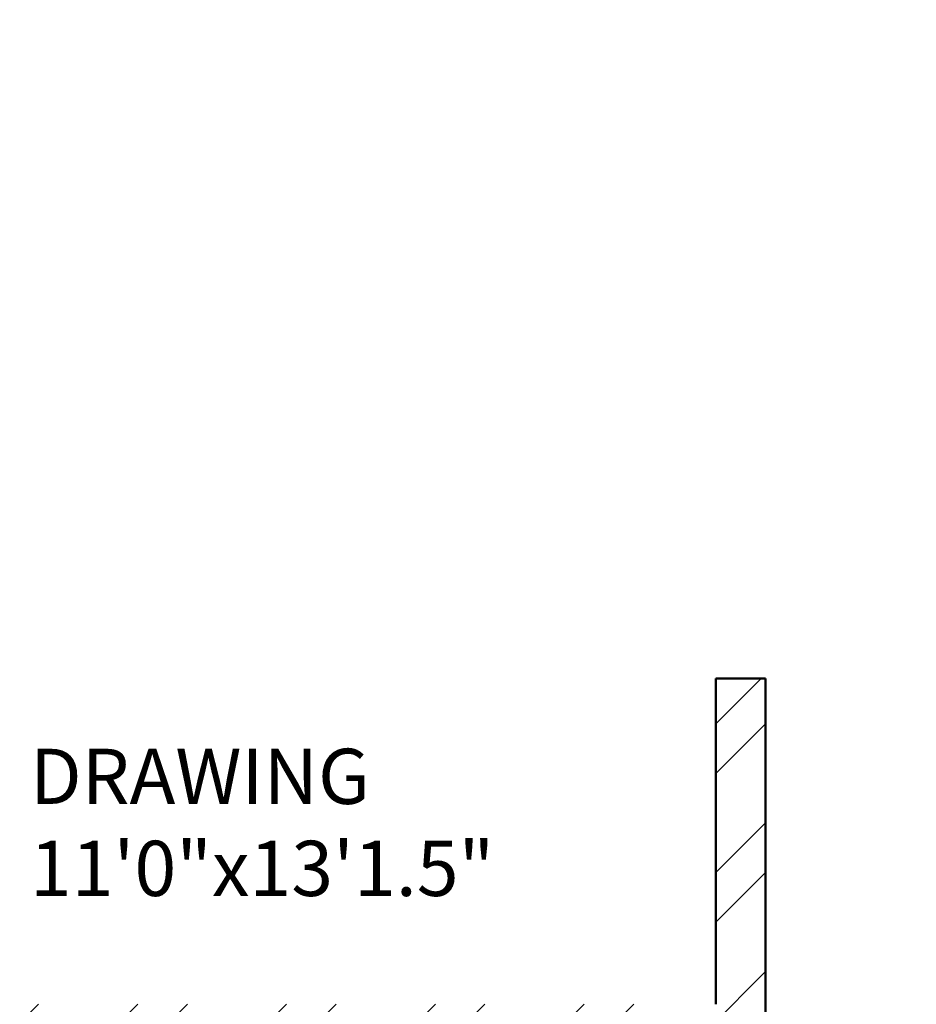
# Model space of a CAD drawing. Units: inches. Extents: x 963 to 2075, y 289 to 2657.
# Tile 53 of 98: x 1582 to 1663, y 1714 to 1803. Entities that reach past the tile are written whole.
import ezdxf

# ---------------------------------------------------------------- set-up
doc = ezdxf.new("R2010")
doc.units = ezdxf.units.IN
for name, color, linetype, lineweight in [('A-AREA-IDEN', 7, 'Continuous', 18), ('A-WALL', 7, 'Continuous', 50), ('A-WALL-PATT', 8, 'Continuous', 13)]:
    doc.layers.add(name, color=color, linetype=linetype, lineweight=lineweight)
doc.styles.get("Standard").update_dxf_attribs({"font": 'arial.ttf'})

msp = doc.modelspace()

# ---------------------------------------------------------------- hatches: boundary and pattern name
at = {"layer": 'A-WALL-PATT'}
h = msp.add_hatch(dxfattribs=at)
h.set_pattern_fill('ANSI32', color=256)
h.paths.add_polyline_path([(1473.609, 2163.068), (1473.609, 2165.318), (1376.422, 2165.318), (1376.422, 2227.983), (1371.922, 2227.983), (1371.922, 2214.818), (1368.405, 2214.818), (1368.405, 2210.318), (1371.922, 2210.318), (1371.922, 2160.818), (1395.922, 2160.818), (1395.922, 2090.318), (1217.345, 2090.318), (1217.345, 2085.818), (1395.922, 2085.818), (1458.922, 2085.818), (1458.922, 2108.318), (1454.422, 2108.318), (1454.422, 2090.318), (1400.422, 2090.318), (1400.422, 2160.818), (1473.609, 2160.818)])
h.paths.add_polyline_path([(1649.422, 2210.318), (1653.225, 2210.318), (1653.225, 2214.818), (1649.422, 2214.818), (1649.422, 2227.983), (1644.922, 2227.983), (1644.922, 2165.318), (1550.099, 2165.318), (1550.099, 2160.818), (1620.922, 2160.818), (1620.922, 2112.818), (1555.446, 2112.818), (1555.446, 2108.318), (1584.327, 2108.318), (1584.327, 2084.916), (1588.827, 2084.916), (1588.827, 2108.318), (1625.422, 2108.318), (1667.951, 2108.318), (1667.951, 2022.667), (1588.827, 2022.667), (1588.827, 2047.408), (1584.327, 2047.408), (1584.327, 1996.003), (1588.827, 1996.003), (1588.827, 2018.318), (1667.951, 2018.167), (1667.951, 1928.318), (1625.422, 1928.318), (1625.422, 1923.818), (1672.451, 1923.818), (1672.451, 1928.318), (1672.451, 1946.663), (1785.446, 1946.663), (1785.446, 1951.163), (1743.034, 1951.163), (1743.034, 2017.922), (1841.422, 2017.922), (1841.422, 2014.775), (1845.922, 2014.775), (1845.922, 2017.922), (1905.922, 2017.922), (1905.922, 1987.511), (1910.422, 1987.511), (1910.422, 2022.422), (1910.422, 2068.517), (1905.922, 2068.517), (1905.922, 2022.422), (1845.922, 2022.422), (1845.922, 2025.851), (1843.672, 2025.851), (1841.422, 2025.851), (1841.422, 2022.422), (1743.034, 2022.422), (1743.034, 2084.031), (1768.451, 2084.031), (1785.446, 2084.031), (1785.446, 2088.531), (1672.451, 2088.531), (1672.451, 2112.818), (1667.951, 2112.818), (1625.422, 2112.818), (1625.422, 2160.818), (1649.422, 2160.818)])
h.paths.add_polyline_path([(1672.451, 2084.031), (1738.534, 2084.031), (1738.534, 1951.163), (1672.451, 1951.163)], flags=16)
h.paths.add_polyline_path([(1672.451, 2084.031), (1738.534, 2084.031), (1705.492, 2017.597)], flags=0)
h.paths.add_polyline_path([(1262.766, 2085.818), (1258.266, 2085.818), (1258.266, 2023.278), (1184.422, 2023.278), (1184.422, 2018.778), (1258.266, 2018.778), (1258.266, 1950.818), (1262.766, 1950.818)])
h.paths.add_polyline_path([(1312.266, 2085.818), (1307.766, 2085.818), (1307.766, 1950.818), (1312.266, 1950.818)])
h.paths.add_polyline_path([(1458.922, 1950.818), (1395.922, 1950.818), (1216.568, 1950.818), (1216.568, 1946.318), (1346.422, 1946.318), (1395.922, 1946.318), (1395.922, 1875.818), (1371.922, 1875.818), (1371.922, 1826.318), (1368.931, 1826.318), (1368.931, 1821.818), (1371.922, 1821.818), (1371.922, 1813.622), (1376.422, 1813.622), (1376.422, 1871.318), (1474.504, 1871.318), (1474.504, 1873.568), (1474.504, 1875.818), (1400.422, 1875.818), (1400.422, 1946.318), (1454.422, 1946.318), (1454.422, 1928.318), (1458.922, 1928.318)])
h.paths.add_polyline_path([(1184.422, 2120.778), (1167.922, 2120.778), (1167.922, 2134.812), (1165.672, 2134.812), (1163.422, 2134.812), (1163.422, 2120.778), (1119.922, 2120.778), (1119.922, 2098.095), (1124.422, 2098.095), (1124.422, 2116.278), (1167.922, 2116.278), (1179.922, 2116.278), (1179.922, 2045.916), (1184.422, 2045.916), (1184.422, 2090.318), (1184.422, 2116.278)])
h.paths.add_polyline_path([(1124.422, 2018.778), (1179.922, 2018.778), (1179.922, 2016.294), (1184.422, 2016.294), (1184.422, 2023.278), (1184.422, 2026.588), (1182.172, 2026.588), (1179.922, 2026.588), (1179.922, 2023.278), (1124.422, 2023.278), (1124.422, 2074.095), (1119.922, 2074.095), (1119.922, 2018.778), (1119.922, 1979.633), (1124.422, 1979.633)])
h.paths.add_polyline_path([(1184.422, 1925.778), (1184.422, 1946.318), (1184.422, 1996.073), (1182.172, 1996.073), (1179.922, 1996.073), (1179.922, 1925.778), (1124.422, 1925.778), (1124.422, 1955.633), (1119.922, 1955.502), (1119.922, 1921.278), (1158.922, 1921.278), (1158.922, 1909.983), (1163.422, 1909.983), (1163.422, 1921.278), (1184.422, 1921.278)])
h.paths.add_polyline_path([(1341.449, 1826.318), (1163.422, 1826.318), (1163.422, 1849.983), (1158.922, 1849.983), (1158.922, 1821.818), (1158.922, 1804.033), (1163.422, 1804.033), (1163.422, 1821.818), (1341.449, 1821.818)])
h.paths.add_polyline_path([(1222.981, 1713.818), (1163.422, 1713.818), (1163.422, 1744.033), (1161.172, 1744.033), (1158.922, 1744.033), (1158.922, 1713.818), (1119.922, 1713.818), (1119.922, 1694.65), (1124.422, 1694.65), (1124.422, 1709.318), (1158.922, 1709.318), (1222.981, 1709.318)])
h.paths.add_polyline_path([(1328.422, 1713.818), (1252.042, 1713.818), (1252.042, 1711.568), (1252.042, 1709.318), (1256.422, 1709.318), (1256.422, 1547.318), (1232.937, 1547.318), (1232.937, 1545.068), (1232.937, 1542.818), (1292.422, 1542.818), (1292.422, 1527.634), (1296.922, 1527.634), (1296.922, 1542.818), (1299.464, 1542.818), (1299.464, 1547.318), (1260.922, 1547.318), (1260.922, 1658.318), (1343.661, 1658.318), (1343.661, 1660.568), (1343.661, 1662.818), (1328.422, 1662.818), (1328.422, 1676.589), (1327.402, 1676.589), (1323.922, 1676.589), (1323.922, 1662.818), (1260.922, 1662.818), (1260.922, 1709.318), (1323.922, 1709.318), (1323.922, 1699.851), (1328.422, 1699.851)])
h.paths.add_polyline_path([(1649.422, 1875.818), (1625.422, 1875.818), (1625.422, 1928.318), (1620.922, 1928.318), (1588.827, 1928.318), (1588.827, 1950.59), (1584.327, 1950.59), (1584.327, 1928.318), (1555.446, 1928.318), (1555.446, 1923.818), (1620.922, 1923.818), (1620.922, 1875.818), (1548.952, 1875.818), (1548.952, 1873.568), (1548.952, 1871.318), (1644.922, 1871.318), (1644.922, 1813.622), (1649.422, 1813.622), (1649.422, 1821.818), (1652.045, 1821.818), (1652.045, 1824.068), (1652.045, 1826.318), (1649.422, 1826.318)])
h.paths.add_polyline_path([(1512.922, 1871.318), (1516.476, 1871.318), (1516.476, 1875.818), (1512.922, 1875.818), (1512.922, 1923.818), (1512.922, 1928.318), (1512.922, 1930.827), (1508.422, 1930.827), (1508.422, 1875.818), (1504.411, 1875.818), (1504.411, 1871.318), (1508.422, 1871.318), (1508.422, 1713.818), (1376.422, 1713.818), (1376.422, 1743.325), (1371.922, 1743.325), (1371.922, 1709.318), (1371.922, 1706.01), (1376.422, 1706.01), (1376.422, 1709.318), (1508.422, 1709.318), (1508.422, 1547.318), (1501.871, 1547.318), (1501.871, 1542.818), (1508.422, 1542.818), (1508.422, 1482.818), (1508.422, 1436.318), (1512.922, 1436.318), (1512.922, 1542.818), (1519.318, 1542.818), (1519.318, 1545.068), (1519.318, 1547.318), (1512.922, 1547.318), (1512.922, 1709.318), (1644.922, 1709.318), (1644.922, 1707.548), (1649.422, 1707.548), (1649.422, 1709.318), (1649.422, 1743.325), (1644.922, 1743.325), (1644.922, 1713.818), (1512.922, 1713.818)])
h.paths.add_polyline_path([(1129.884, 1545.068), (1129.884, 1547.318), (1124.422, 1547.318), (1095.922, 1547.318), (1095.922, 1614.818), (1124.422, 1614.818), (1124.422, 1619.318), (1095.922, 1619.318), (1091.422, 1619.318), (1091.422, 1542.818), (1095.922, 1542.818), (1119.922, 1542.818), (1129.884, 1542.818)])
h.paths.add_polyline_path([(1208.422, 1542.818), (1211.74, 1542.818), (1211.74, 1547.318), (1198.851, 1547.318), (1198.851, 1542.818), (1203.922, 1542.818), (1203.922, 1478.318), (1208.422, 1478.318), (1296.922, 1478.318), (1296.922, 1503.634), (1292.422, 1503.634), (1292.422, 1482.818), (1208.422, 1482.818)])
h.paths.add_polyline_path([(1430.422, 1542.818), (1435.699, 1542.818), (1435.699, 1545.068), (1435.699, 1547.318), (1422.658, 1547.318), (1422.658, 1545.068), (1422.658, 1542.818), (1425.922, 1542.818), (1425.922, 1482.857), (1341.922, 1482.857), (1341.922, 1502.732), (1337.422, 1502.732), (1337.422, 1478.357), (1425.922, 1478.357), (1425.922, 1440.818), (1425.922, 1436.318), (1430.422, 1436.318)])
h.paths.add_polyline_path([(1698.482, 2004.259), (1727.695, 2004.259), (1727.695, 2022.916), (1698.482, 2022.916)], flags=8)

# ---------------------------------------------------------------- linework, layer by layer
at = {"layer": 'A-WALL'}
for p, q in [((1644.922, 1713.818), (1644.922, 1743.325)), ((1644.922, 1743.325), (1649.422, 1743.325)), ((1649.422, 1709.318), (1649.422, 1743.325))]:
    msp.add_line(p, q, dxfattribs=at)

# ---------------------------------------------------------------- texts
at = {"layer": 'A-AREA-IDEN', "insert": (1582.81, 1736.962), "char_height": 5, "attachment_point": 1}
msp.add_mtext_dynamic_manual_height_columns('DRAWING\\P11\'0"x13\'1.5"', width=162.25013, gutter_width=12.5, heights=[0], dxfattribs=at)

doc.saveas('drawing.dxf')
